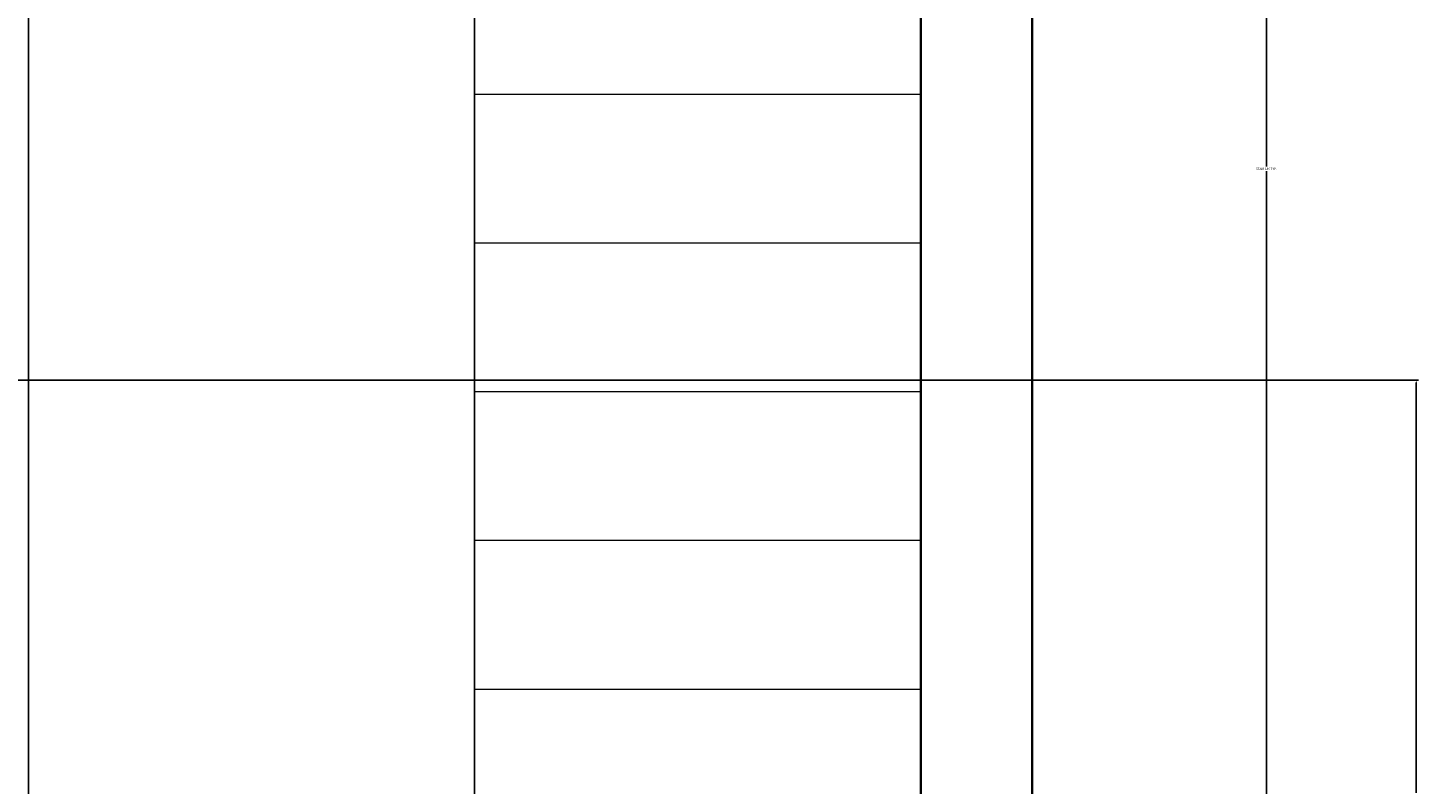
# Model space of a CAD drawing. Units: feet. Extents: x 1654 to 2985, y 1348 to 2230.
# Tile 22 of 53: x 2130 to 2242, y 1609 to 1670. Entities that reach past the tile are written whole.
import ezdxf

# ---------------------------------------------------------------- set-up
doc = ezdxf.new("R2010")
doc.units = ezdxf.units.FT
for name, color, linetype, lineweight in [('A-ANNO-DIMS', 2, 'Continuous', 18), ('A-FLOR-STRS', 7, 'Continuous', 18), ('A-WALL', 7, 'Continuous', 35)]:
    doc.layers.add(name, color=color, linetype=linetype, lineweight=lineweight)
doc.styles.get("Standard").update_dxf_attribs({"font": 'arial.ttf'})
doc.dimstyles.get("Standard").update_dxf_attribs({"dimtxt": 0.18, "dimasz": 0.18, "dimexe": 0.18, "dimexo": 0.0625, "dimgap": 0.09, "dimtad": 0, "dimtih": 1, "dimtoh": 1, "dimdec": 4, "dimzin": 0, "dimdsep": 46, "dimtxsty": 'Standard', "dimcen": 0.09, "dimadec": 0, "dimazin": 0, "dimtfac": 1, "dimtdec": 4, "dimtofl": 0, "dimtmove": 0, "dimatfit": 3, "dimfxl": 1, "dimtolj": 1, "dimtzin": 0, "dimarcsym": 0})

# ---------------------------------------------------------------- blocks, each defined once
blk = doc.blocks.new('STAIR-RETURN')
for p, q in [((36, 186), (36, 0)), ((72, 99), (36, 99)), ((72, 87), (36, 87)), ((72, 75), (36, 75)), ((72, 63), (36, 63)), ((72, 51), (36, 51))]:
    blk.add_line(p, q)
blk = doc.blocks.new('*D72')
at = {"layer": 'A-ANNO-DIMS', "color": 0, "lineweight": -2, "transparency": 16777216}
for p, q in [((2202.15, 1751.25), (2230.17, 1751.25)), ((2229.99, 1751.07), (2229.99, 1658.44)), ((2229.99, 1565.43), (2229.99, 1658.07)), ((2202.15, 1565.25), (2230.17, 1565.25))]:
    blk.add_line(p, q, dxfattribs=at)
at = {"layer": 'A-ANNO-DIMS', "color": 0, "transparency": 16777216}
for points in [[(2229.96, 1751.07), (2230.02, 1751.07), (2229.99, 1751.25)], [(2229.96, 1565.43), (2230.02, 1565.43), (2229.99, 1565.25)]]:
    blk.add_solid(points, dxfattribs=at)
at = {"layer": 'Defpoints', "color": 0, "transparency": 16777216}
for p in [(2202.09, 1751.25), (2229.99, 1751.25), (2202.09, 1565.25)]:
    blk.add_point(p, dxfattribs=at)
at = {"layer": 'A-ANNO-DIMS', "color": 0, "transparency": 16777216, "insert": (2229.99, 1658.25), "char_height": 0.18, "attachment_point": 5}
blk.add_mtext('\\A1;STAIR 186 TYP.', dxfattribs=at)
blk = doc.blocks.new('*D80')
at = {"layer": 'A-ANNO-DIMS', "color": 0, "lineweight": -2, "transparency": 16777216}
for p, q in [((2070.09, 2039.19), (2070.09, 1534.07)), ((2202.09, 2039.19), (2202.09, 1534.07)), ((2070.27, 1534.25), (2135.81, 1534.25)), ((2201.91, 1534.25), (2136.37, 1534.25))]:
    blk.add_line(p, q, dxfattribs=at)
at = {"layer": 'A-ANNO-DIMS', "color": 0, "transparency": 16777216}
for points in [[(2070.27, 1534.28), (2070.27, 1534.22), (2070.09, 1534.25)], [(2201.91, 1534.28), (2201.91, 1534.22), (2202.09, 1534.25)]]:
    blk.add_solid(points, dxfattribs=at)
at = {"layer": 'Defpoints', "color": 0, "transparency": 16777216}
for p in [(2070.09, 2039.25), (2202.09, 2039.25), (2202.09, 1534.25)]:
    blk.add_point(p, dxfattribs=at)
at = {"layer": 'A-ANNO-DIMS', "color": 0, "transparency": 16777216, "insert": (2136.09, 1534.25), "char_height": 0.18, "attachment_point": 5}
blk.add_mtext('\\A1;132', dxfattribs=at)
blk = doc.blocks.new('*D90')
at = {"layer": 'A-ANNO-DIMS', "color": 0, "lineweight": -2, "transparency": 16777216}
for p, q in [((1852.15, 1641.19), (2242.27, 1641.19)), ((2242.09, 1641.01), (2242.09, 1607.9)), ((2242.09, 1574.43), (2242.09, 1607.54)), ((1852.15, 1574.25), (2242.27, 1574.25))]:
    blk.add_line(p, q, dxfattribs=at)
at = {"layer": 'A-ANNO-DIMS', "color": 0, "transparency": 16777216}
for points in [[(2242.06, 1641.01), (2242.12, 1641.01), (2242.09, 1641.19)], [(2242.06, 1574.43), (2242.12, 1574.43), (2242.09, 1574.25)]]:
    blk.add_solid(points, dxfattribs=at)
at = {"layer": 'Defpoints', "color": 0, "transparency": 16777216}
for p in [(1852.09, 1641.19), (2242.09, 1641.19), (1852.09, 1574.25)]:
    blk.add_point(p, dxfattribs=at)
at = {"layer": 'A-ANNO-DIMS', "color": 0, "transparency": 16777216, "insert": (2242.09, 1607.72), "char_height": 0.18, "attachment_point": 5}
blk.add_mtext('\\A1;66.93', dxfattribs=at)
blk = doc.blocks.new('*D99')
at = {"layer": 'A-ANNO-DIMS', "color": 0, "lineweight": -2, "transparency": 16777216}
for p, q in [((2166.09, 1746.69), (2166.09, 1534.07)), ((2130.09, 1742.19), (2130.09, 1534.07)), ((2130.27, 1534.25), (2147.87, 1534.25)), ((2165.91, 1534.25), (2148.31, 1534.25))]:
    blk.add_line(p, q, dxfattribs=at)
at = {"layer": 'A-ANNO-DIMS', "color": 0, "transparency": 16777216}
for points in [[(2130.27, 1534.28), (2130.27, 1534.22), (2130.09, 1534.25)], [(2165.91, 1534.28), (2165.91, 1534.22), (2166.09, 1534.25)]]:
    blk.add_solid(points, dxfattribs=at)
at = {"layer": 'Defpoints', "color": 0, "transparency": 16777216}
for p in [(2166.09, 1746.75), (2130.09, 1742.25), (2166.09, 1534.25)]:
    blk.add_point(p, dxfattribs=at)
at = {"layer": 'A-ANNO-DIMS', "color": 0, "transparency": 16777216, "insert": (2148.09, 1534.25), "char_height": 0.18, "attachment_point": 5}
blk.add_mtext('\\A1;36', dxfattribs=at)
blk = doc.blocks.new('*D103')
at = {"layer": 'A-ANNO-DIMS', "color": 0, "lineweight": -2, "transparency": 16777216}
for p, q in [((2070.09, 1661.19), (2070.09, 1534.07)), ((2130.09, 1565.19), (2130.09, 1534.07)), ((2070.27, 1534.25), (2099.87, 1534.25)), ((2129.91, 1534.25), (2100.31, 1534.25))]:
    blk.add_line(p, q, dxfattribs=at)
at = {"layer": 'A-ANNO-DIMS', "color": 0, "transparency": 16777216}
for points in [[(2070.27, 1534.28), (2070.27, 1534.22), (2070.09, 1534.25)], [(2129.91, 1534.28), (2129.91, 1534.22), (2130.09, 1534.25)]]:
    blk.add_solid(points, dxfattribs=at)
at = {"layer": 'Defpoints', "color": 0, "transparency": 16777216}
for p in [(2070.09, 1661.25), (2130.09, 1565.25), (2130.09, 1534.25)]:
    blk.add_point(p, dxfattribs=at)
at = {"layer": 'A-ANNO-DIMS', "color": 0, "transparency": 16777216, "insert": (2100.09, 1534.25), "char_height": 0.18, "attachment_point": 5}
blk.add_mtext('\\A1;60', dxfattribs=at)

msp = doc.modelspace()

# ---------------------------------------------------------------- linework, layer by layer
at = {"layer": 'A-WALL'}
for p, q in [((2211.0924, 1886.2549), (2211.0924, 1565.2549)), ((2202.0924, 1742.2549), (2202.0924, 1565.2549))]:
    msp.add_line(p, q, dxfattribs=at)

# ---------------------------------------------------------------- block references
at = {"layer": 'A-FLOR-STRS'}
msp.add_blockref('STAIR-RETURN', (2130.092, 1565.255), dxfattribs=at)

# ---------------------------------------------------------------- dimensions: what is measured, and where the dimension line sits
at = {"layer": 'A-ANNO-DIMS'}
for base, p1, p2, picture, middle in [((2202.0924, 1534.2549), (2070.0924, 2039.2549), (2202.0924, 2039.2549), '*D80', (2136.0924, 1534.2549)), ((2166.0924, 1534.2549), (2130.0924, 1742.2549), (2166.0924, 1746.7549), '*D99', (2148.0924, 1534.2549)), ((2130.0924, 1534.2549), (2070.0924, 1661.2549), (2130.0924, 1565.2549), '*D103', (2100.0924, 1534.2549))]:
    dim = msp.add_linear_dim(base=base, p1=p1, p2=p2, dimstyle='Standard', override={"dimdec": 0, "dimlfac": 1, "dimrnd": 0, "dimzin": 0, "dimdsep": 46, "dimlunit": 2}, dxfattribs=at)
    dim.commit()
    dim.dimension.update_dxf_attribs({"geometry": picture, "text_midpoint": middle})
dim = msp.add_linear_dim(base=(2229.9924, 1751.2549), p1=(2202.0924, 1565.2549), p2=(2202.0924, 1751.2549), angle=90, text='STAIR <> TYP.', dimstyle='Standard', override={"dimdec": 0, "dimlfac": 1, "dimrnd": 0, "dimzin": 0, "dimdsep": 46, "dimlunit": 2}, dxfattribs=at)
dim.commit()
dim.dimension.update_dxf_attribs({"geometry": '*D72', "text_midpoint": (2229.9924, 1658.2549)})
dim = msp.add_linear_dim(base=(2242.0924, 1641.187), p1=(1852.0924, 1574.2549), p2=(1852.0924, 1641.187), angle=90, dimstyle='Standard', override={"dimdec": 2, "dimlfac": 1, "dimrnd": 0, "dimzin": 0, "dimdsep": 46, "dimlunit": 2}, dxfattribs=at)
dim.commit()
dim.dimension.update_dxf_attribs({"geometry": '*D90', "text_midpoint": (2242.0924, 1607.721)})

doc.saveas('drawing.dxf')
